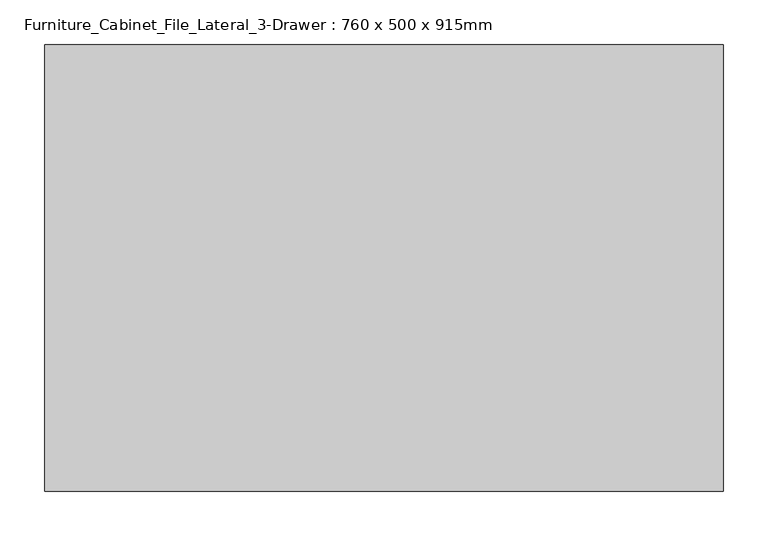
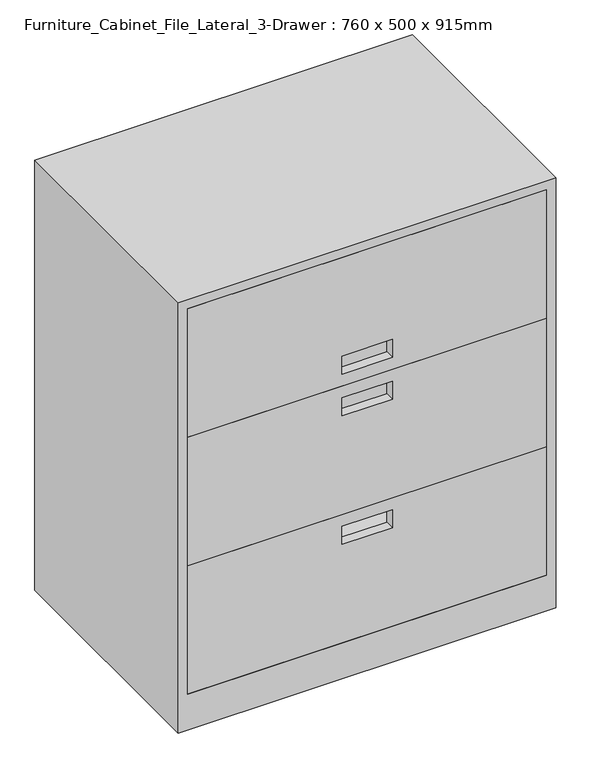
"""IFC4 building model written with IfcOpenShell, lengths in millimetres: furniture geometry, Furniture_Cabinet_File_Lateral_3-Drawer : 760 x 500 x 915mm."""

from ifc_helpers import new_model, si_unit, frame, origin, place, context, project, spatial, polyline, outline, extrude, faceted_brep, source, transform, mapped, element, save


def furniture_cabinet_file_lateral_3_drawer_760_x_500_x_915mm_92c95d2d(model_context):
    return source(origin(), model_context, "Body", "SolidModel", [
        faceted_brep([(199.9774861, -684.3183761, 915.0), (-560.0225139, -684.3183761, 915.0), (-560.0225139, -1184.3183761, 915.0), (199.9774861, -1184.3183761, 915.0), (199.9774861, -684.3183761, 0.0), (199.9774861, -1184.3183761, 0.0), (-560.0225139, -1184.3183761, 0.0), (-560.0225139, -684.3183761, 0.0), (180.9274861, -1184.3183761, 76.2), (-540.9725139, -1184.3183761, 76.2), (-540.9725139, -1184.3183761, 895.95), (180.9274861, -1184.3183761, 895.95), (-540.9725139, -703.3683761, 76.2), (180.9274861, -703.3683761, 76.2), (180.9274861, -703.3683761, 895.95), (-540.9725139, -703.3683761, 895.95)], [[[0, 1, 2, 3]], [[4, 5, 6, 7]], [[1, 0, 4, 7]], [[2, 1, 7, 6]], [[3, 2, 6, 5], [8, 9, 10, 11]], [[0, 3, 5, 4]], [[12, 13, 14, 15]], [[13, 12, 9, 8]], [[14, 13, 8, 11]], [[15, 14, 11, 10]], [[12, 15, 10, 9]]]),
        extrude(outline(polyline([(895.95, -540.9725139), (622.6999998, -540.9725139), (622.7, 180.9274861), (895.95, 180.9274861), (895.95, -540.9725139)]), holes=[polyline([(686.2, -230.8225139), (686.2, -129.2225139), (648.1, -129.2225139), (648.1, -230.8225139), (686.2, -230.8225139)])]), frame((0.0, -1184.3183761, 0.0), z_axis=(0.0, 1.0, 0.0), x_axis=(0.0, 0.0, 1.0)), (0.0, 0.0, 1.0), 19.05),
        extrude(outline(polyline([(349.45, -540.9725139), (349.45, 180.9274861), (622.7, 180.9274861), (622.6999998, -540.9725139), (349.45, -540.9725139)]), holes=[polyline([(597.3, -230.8225139), (597.3, -129.2225139), (559.2, -129.2225139), (559.2, -230.8225139), (597.3, -230.8225139)])]), frame((0.0, -1184.3183761, 0.0), z_axis=(0.0, 1.0, 0.0), x_axis=(0.0, 0.0, 1.0)), (0.0, 0.0, 1.0), 19.05),
        extrude(outline(polyline([(76.2, -540.9725139), (76.2, 180.9274861), (349.45, 180.9274861), (349.45, -540.9725139), (76.2, -540.9725139)]), holes=[polyline([(324.05, -230.8225139), (324.05, -129.2225139), (285.95, -129.2225139), (285.95, -230.8225139), (324.05, -230.8225139)])]), frame((0.0, -1184.3183761, 0.0), z_axis=(0.0, 1.0, 0.0), x_axis=(0.0, 0.0, 1.0)), (0.0, 0.0, 1.0), 19.05),
    ])


if __name__ == "__main__":
    model = new_model("IFC4")
    model_context = context("Model", 3, world=origin())
    ifc_project = project(units=[si_unit("LENGTHUNIT", "METRE", prefix="MILLI")], contexts=[model_context])
    site = spatial("IfcSite", under=ifc_project)
    building = spatial("IfcBuilding", under=site)
    placement = place(None, origin())
    furniture_cabinet_file_lateral_3_drawer_760_x_500_x_915mm_shape = furniture_cabinet_file_lateral_3_drawer_760_x_500_x_915mm_92c95d2d(model_context)
    element("IfcFurniture", 1, ObjectType="Furniture_Cabinet_File_Lateral_3-Drawer : 760 x 500 x 915mm", at=placement, inside=building, context=model_context, shape_type="MappedRepresentation", body=[
        mapped(furniture_cabinet_file_lateral_3_drawer_760_x_500_x_915mm_shape, transform((0.0, 0.0, 0.0), x_axis=(1.0, 0.0, 0.0), y_axis=(0.0, 1.0, 0.0), z_axis=(0.0, 0.0, 1.0))),
    ])
    save(model, "model.ifc")

# Revit data of these elements
# Type "Furniture_Cabinet_File_Lateral_3-Drawer : 760 x 500 x 915mm"
#   Keynote = "N"
#   Depth = 1' - 7.68504"
#   Height = 3' - 0.02362"
#   Width = 2' - 5.92126"
#   Material = Metal - Steel
#   Default Elevation = 0
#   Assembly Code = ""
# Element 1 (IfcFurniture, "Furniture_Cabinet_File_Lateral_3-Drawer : 760 x 500 x 915mm")
#   Materials on its faces: "Metal - Steel"
# Materials
#   "Metal - Steel": class "Metal", colour RGB 209 209 209, transparency 0
